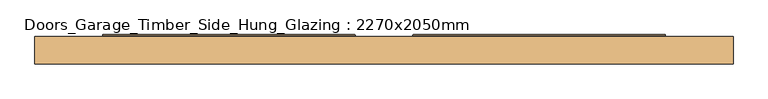
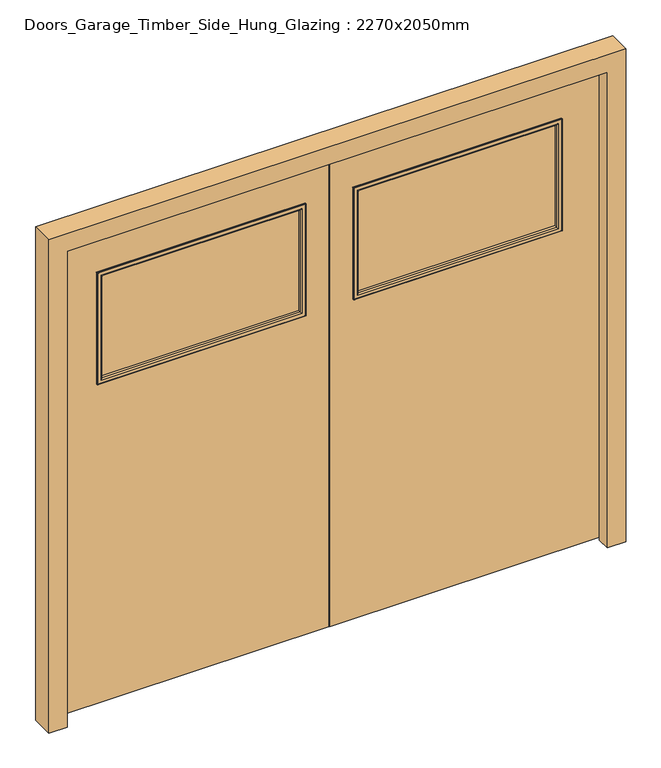
"""IFC4 building model written with IfcOpenShell, lengths in millimetres: door geometry, Doors_Garage_Timber_Side_Hung_Glazing : 2270x2050mm."""

from ifc_helpers import new_model, si_unit, frame, origin, place, context, project, spatial, polyline, ellipse_curve, outline, extrude, faceted_brep, source, transform, mapped, element, save
from ifc_brep_helpers import plane_surface, cylinder_surface, advanced_brep


def doors_garage_timber_side_hung_glazing_2270x2050mm_ae99176d(model_context):
    return source(origin(), model_context, "Body", "SolidModel", [
        faceted_brep([(1085.0, 76.6, 0.0), (1135.0, 76.6, 0.0), (1135.0, -12.4, 0.0), (1063.0, -12.4, 0.0), (1063.0, 41.6, 0.0), (1085.0, 41.6, 0.0), (1085.0, 76.6, 2000.0), (-1085.0, 76.6, 2000.0), (-1085.0, 76.6, 0.0), (-1135.0, 76.6, 0.0), (-1135.0, 76.6, 2050.0), (1135.0, 76.6, 2050.0), (1135.0, -12.4, 2050.0), (-1135.0, -12.4, 2050.0), (-1135.0, -12.4, 0.0), (-1063.0, -12.4, 0.0), (-1063.0, -12.4, 1978.0), (1063.0, -12.4, 1978.0), (1063.0, 41.6, 1978.0), (-1063.0, 41.6, 1978.0), (-1063.0, 41.6, 0.0), (-1085.0, 41.6, 0.0), (-1085.0, 41.6, 2000.0), (1085.0, 41.6, 2000.0)], [[[0, 1, 2, 3, 4, 5]], [[1, 0, 6, 7, 8, 9, 10, 11]], [[2, 1, 11, 12]], [[3, 2, 12, 13, 14, 15, 16, 17]], [[4, 3, 17, 18]], [[5, 4, 18, 19, 20, 21, 22, 23]], [[0, 5, 23, 6]], [[8, 7, 22, 21]], [[9, 8, 21, 20, 15, 14]], [[10, 9, 14, 13]], [[16, 15, 20, 19]], [[11, 10, 13, 12]], [[17, 16, 19, 18]], [[7, 6, 23, 22]]]),
        faceted_brep([(1.5, 44.6, 10.0), (1082.0, 44.6, 10.0), (1082.0, 44.6, 1997.0), (1.5, 44.6, 1997.0), (101.5, 44.6, 1797.0), (907.0, 44.6, 1797.0), (907.0, 44.6, 1347.0), (101.5, 44.6, 1347.0), (1.5, 76.6, 10.0), (1.5, 76.6, 1997.0), (1082.0, 76.6, 1997.0), (1082.0, 76.6, 10.0), (101.5, 76.6, 1797.0), (101.5, 76.6, 1347.0), (907.0, 76.6, 1347.0), (907.0, 76.6, 1797.0), (101.5, 76.6, 1147.0), (101.5, 76.6, 260.0), (907.0, 76.6, 260.0), (907.0, 76.6, 1147.0), (101.5, 71.6, 260.0), (101.5, 71.6, 1147.0), (907.0, 71.6, 1147.0), (907.0, 71.6, 260.0)], [[[0, 1, 2, 3], [4, 5, 6, 7]], [[8, 9, 10, 11], [12, 13, 14, 15], [16, 17, 18, 19]], [[1, 0, 8, 11]], [[2, 1, 11, 10]], [[3, 2, 10, 9]], [[0, 3, 9, 8]], [[5, 4, 12, 15]], [[6, 5, 15, 14]], [[7, 6, 14, 13]], [[4, 7, 13, 12]], [[20, 21, 22, 23]], [[21, 20, 17, 16]], [[22, 21, 16, 19]], [[23, 22, 19, 18]], [[20, 23, 18, 17]]]),
        faceted_brep([(-1082.0, 44.6, 10.0), (-1.5, 44.6, 10.0), (-1.5, 44.6, 1997.0), (-1082.0, 44.6, 1997.0), (-101.5, 44.6, 1347.0), (-907.0, 44.6, 1347.0), (-907.0, 44.6, 1797.0), (-101.5, 44.6, 1797.0), (-1082.0, 76.6, 10.0), (-1082.0, 76.6, 1997.0), (-1.5, 76.6, 1997.0), (-1.5, 76.6, 10.0), (-101.5, 76.6, 1347.0), (-101.5, 76.6, 1797.0), (-907.0, 76.6, 1797.0), (-907.0, 76.6, 1347.0), (-101.5, 76.6, 1147.0), (-907.0, 76.6, 1147.0), (-907.0, 76.6, 260.0), (-101.5, 76.6, 260.0), (-907.0, 71.6, 1147.0), (-101.5, 71.6, 1147.0), (-101.5, 71.6, 260.0), (-907.0, 71.6, 260.0)], [[[0, 1, 2, 3], [4, 5, 6, 7]], [[8, 9, 10, 11], [12, 13, 14, 15], [16, 17, 18, 19]], [[1, 0, 8, 11]], [[2, 1, 11, 10]], [[3, 2, 10, 9]], [[0, 3, 9, 8]], [[5, 4, 12, 15]], [[6, 5, 15, 14]], [[7, 6, 14, 13]], [[4, 7, 13, 12]], [[20, 21, 22, 23]], [[21, 20, 17, 16]], [[22, 21, 16, 19]], [[23, 22, 19, 18]], [[20, 23, 18, 17]]]),
        extrude(outline(polyline([(907.0, 54.6), (101.5, 54.6), (101.5, 66.6), (907.0, 66.6), (907.0, 54.6)])), frame((0.0, 0.0, 1347.0), z_axis=(0.0, 0.0, 1.0), x_axis=(1.0, 0.0, 0.0)), (0.0, 0.0, 1.0), 450.0),
        extrude(outline(polyline([(-101.5, 54.6), (-907.0, 54.6), (-907.0, 66.6), (-101.5, 66.6), (-101.5, 54.6)])), frame((0.0, 0.0, 1347.0), z_axis=(0.0, 0.0, 1.0), x_axis=(1.0, 0.0, 0.0)), (0.0, 0.0, 1.0), 450.0),
        advanced_brep(
        [(-907.0, 66.6, 1797.0), (-907.0, 76.6, 1797.0), (-907.0, 76.6, 1347.0), (-907.0, 66.6, 1347.0), (-895.0, 77.6, 1785.0), (-895.0, 66.6, 1785.0), (-895.0, 66.6, 1359.0), (-895.0, 77.6, 1359.0), (-900.0, 82.6, 1790.0), (-900.0, 82.6, 1354.0), (-915.0, 80.6, 1805.0), (-913.0, 82.6, 1803.0), (-913.0, 82.6, 1341.0), (-915.0, 80.6, 1339.0), (-915.0, 76.6, 1805.0), (-915.0, 76.6, 1339.0), (-101.5, 76.6, 1347.0), (-101.5, 66.6, 1347.0), (-113.5, 66.6, 1359.0), (-113.5, 77.6, 1359.0), (-108.5, 82.6, 1354.0), (-95.5, 82.6, 1341.0), (-93.5, 80.6, 1339.0), (-93.5, 76.6, 1339.0), (-101.5, 76.6, 1797.0), (-101.5, 66.6, 1797.0), (-113.5, 66.6, 1785.0), (-113.5, 77.6, 1785.0), (-108.5, 82.6, 1790.0), (-95.5, 82.6, 1803.0), (-93.5, 80.6, 1805.0), (-93.5, 76.6, 1805.0)],
        [
            (0, 1),
            (1, 2),
            (2, 3),
            (3, 0),
            (4, 5),
            (5, 6),
            (6, 7),
            (7, 4),
            (8, 4, ellipse_curve(frame((-900.0, 77.6, 1790.0), z_axis=(-0.7071067811865475, 0.0, -0.7071067811865475), x_axis=(-0.7071067811865474, 0.0, 0.7071067811865476)), 7.0710678, 5.0)),
            (7, 9, ellipse_curve(frame((-900.0, 77.6, 1354.0), z_axis=(-0.7071067811865475, 0.0, 0.7071067811865475), x_axis=(0.7071067811865474, 0.0, 0.7071067811865476)), 7.0710678, 5.0)),
            (9, 8),
            (10, 11, ellipse_curve(frame((-913.0, 80.6, 1803.0), z_axis=(-0.7071067811865475, 0.0, -0.7071067811865475), x_axis=(-0.7071067811865474, 0.0, 0.7071067811865476)), 2.8284271, 2.0)),
            (11, 12),
            (12, 13, ellipse_curve(frame((-913.0, 80.6, 1341.0), z_axis=(-0.7071067811865475, 0.0, 0.7071067811865475), x_axis=(0.7071067811865474, 0.0, 0.7071067811865476)), 2.8284271, 2.0)),
            (13, 10),
            (14, 10),
            (13, 15),
            (15, 14),
            (2, 16),
            (16, 17),
            (17, 3),
            (6, 18),
            (18, 19),
            (19, 7),
            (19, 20, ellipse_curve(frame((-108.5, 77.6, 1354.0), z_axis=(-0.7071067811865475, 0.0, -0.7071067811865475), x_axis=(-0.7071067811865476, 0.0, 0.7071067811865474)), 7.0710678, 5.0)),
            (20, 9),
            (12, 21),
            (21, 22, ellipse_curve(frame((-95.5, 80.6, 1341.0), z_axis=(-0.7071067811865475, 0.0, -0.7071067811865475), x_axis=(-0.7071067811865476, 0.0, 0.7071067811865474)), 2.8284271, 2.0)),
            (22, 13),
            (22, 23),
            (23, 15),
            (16, 24),
            (24, 25),
            (25, 17),
            (18, 26),
            (26, 27),
            (27, 19),
            (27, 28, ellipse_curve(frame((-108.5, 77.6, 1790.0), z_axis=(0.7071067811865475, 0.0, -0.7071067811865475), x_axis=(-0.7071067811865474, 0.0, -0.7071067811865476)), 7.0710678, 5.0)),
            (28, 20),
            (21, 29),
            (29, 30, ellipse_curve(frame((-95.5, 80.6, 1803.0), z_axis=(0.7071067811865475, 0.0, -0.7071067811865475), x_axis=(-0.7071067811865474, 0.0, -0.7071067811865476)), 2.8284271, 2.0)),
            (30, 22),
            (30, 31),
            (31, 23),
            (31, 14),
            (1, 24),
            (0, 25),
            (5, 26),
            (4, 27),
            (8, 28),
            (11, 29),
            (10, 30),
        ],
        [
            plane_surface(frame((-907.0, 76.6, 1797.0), z_axis=(-1.0, 0.0, 0.0), x_axis=(0.0, 0.0, -1.0))),
            plane_surface(frame((-895.0, 66.6, 1785.0), z_axis=(1.0, 0.0, 0.0), x_axis=(0.0, 0.0, -1.0))),
            cylinder_surface(frame((-900.0, 77.6, 1797.0), z_axis=(0.0, 0.0, 1.0), x_axis=(-1.0, 0.0, 0.0)), 5.0),
            cylinder_surface(frame((-913.0, 80.6, 1797.0), z_axis=(0.0, 0.0, 1.0), x_axis=(-1.0, 0.0, 0.0)), 2.0),
            plane_surface(frame((-915.0, 80.6, 1805.0), z_axis=(-1.0, 0.0, 0.0), x_axis=(0.0, 0.0, -1.0))),
            plane_surface(frame((-907.0, 76.6, 1347.0), z_axis=(0.0, 0.0, -1.0), x_axis=(1.0, 0.0, 0.0))),
            plane_surface(frame((-895.0, 66.6, 1359.0), z_axis=(0.0, 0.0, 1.0), x_axis=(1.0, 0.0, 0.0))),
            cylinder_surface(frame((-907.0, 77.6, 1354.0), z_axis=(-1.0, 0.0, 0.0), x_axis=(0.0, 0.0, -1.0)), 5.0),
            cylinder_surface(frame((-907.0, 80.6, 1341.0), z_axis=(-1.0, 0.0, 0.0), x_axis=(0.0, 0.0, -1.0)), 2.0),
            plane_surface(frame((-915.0, 80.6, 1339.0), z_axis=(0.0, 0.0, -1.0), x_axis=(1.0, 0.0, 0.0))),
            plane_surface(frame((-101.5, 76.6, 1347.0), z_axis=(1.0, 0.0, 0.0), x_axis=(0.0, 0.0, 1.0))),
            plane_surface(frame((-113.5, 66.6, 1359.0), z_axis=(-1.0, 0.0, 0.0), x_axis=(0.0, 0.0, 1.0))),
            cylinder_surface(frame((-108.5, 77.6, 1347.0), z_axis=(0.0, 0.0, -1.0), x_axis=(1.0, 0.0, 0.0)), 5.0),
            cylinder_surface(frame((-95.5, 80.6, 1347.0), z_axis=(0.0, 0.0, -1.0), x_axis=(1.0, 0.0, 0.0)), 2.0),
            plane_surface(frame((-93.5, 80.6, 1339.0), z_axis=(1.0, 0.0, 0.0), x_axis=(0.0, 0.0, 1.0))),
            plane_surface(frame((-93.5, 76.6, 1805.0), z_axis=(0.0, -1.0, 0.0), x_axis=(-1.0, 0.0, 0.0))),
            plane_surface(frame((-101.5, 76.6, 1797.0), z_axis=(0.0, 0.0, 1.0), x_axis=(-1.0, 0.0, 0.0))),
            plane_surface(frame((-101.5, 66.6, 1797.0), z_axis=(0.0, -1.0, 0.0), x_axis=(-1.0, 0.0, 0.0))),
            plane_surface(frame((-113.5, 66.6, 1785.0), z_axis=(0.0, 0.0, -1.0), x_axis=(-1.0, 0.0, 0.0))),
            cylinder_surface(frame((-101.5, 77.6, 1790.0), z_axis=(1.0, 0.0, 0.0), x_axis=(0.0, 0.0, 1.0)), 5.0),
            plane_surface(frame((-108.5, 82.6, 1790.0), z_axis=(0.0, 1.0, 0.0), x_axis=(-1.0, 0.0, 0.0))),
            cylinder_surface(frame((-101.5, 80.6, 1803.0), z_axis=(1.0, 0.0, 0.0), x_axis=(0.0, 0.0, 1.0)), 2.0),
            plane_surface(frame((-93.5, 80.6, 1805.0), z_axis=(0.0, 0.0, 1.0), x_axis=(-1.0, 0.0, 0.0))),
        ],
        [
            (0, [[1, 2, 3, 4]]),
            (1, [[5, 6, 7, 8]]),
            (2, [[9, -8, 10, 11]]),
            (3, [[12, 13, 14, 15]]),
            (4, [[16, -15, 17, 18]]),
            (5, [[-3, 19, 20, 21]]),
            (6, [[-7, 22, 23, 24]]),
            (7, [[-10, -24, 25, 26]]),
            (8, [[-14, 27, 28, 29]]),
            (9, [[-17, -29, 30, 31]]),
            (10, [[-20, 32, 33, 34]]),
            (11, [[-23, 35, 36, 37]]),
            (12, [[-25, -37, 38, 39]]),
            (13, [[-28, 40, 41, 42]]),
            (14, [[-30, -42, 43, 44]]),
            (15, [[-31, -44, 45, -18], [46, -32, -19, -2]]),
            (16, [[-33, -46, -1, 47]]),
            (17, [[-21, -34, -47, -4], [48, -35, -22, -6]]),
            (18, [[-36, -48, -5, 49]]),
            (19, [[-38, -49, -9, 50]]),
            (20, [[51, -40, -27, -13], [-26, -39, -50, -11]]),
            (21, [[-41, -51, -12, 52]]),
            (22, [[-43, -52, -16, -45]]),
        ],
    ),
        advanced_brep(
        [(101.5, 66.6, 1797.0), (101.5, 76.6, 1797.0), (101.5, 76.6, 1347.0), (101.5, 66.6, 1347.0), (113.5, 77.6, 1785.0), (113.5, 66.6, 1785.0), (113.5, 66.6, 1359.0), (113.5, 77.6, 1359.0), (108.5, 82.6, 1790.0), (108.5, 82.6, 1354.0), (93.5, 80.6, 1805.0), (95.5, 82.6, 1803.0), (95.5, 82.6, 1341.0), (93.5, 80.6, 1339.0), (93.5, 76.6, 1805.0), (93.5, 76.6, 1339.0), (907.0, 76.6, 1347.0), (907.0, 66.6, 1347.0), (895.0, 66.6, 1359.0), (895.0, 77.6, 1359.0), (900.0, 82.6, 1354.0), (913.0, 82.6, 1341.0), (915.0, 80.6, 1339.0), (915.0, 76.6, 1339.0), (907.0, 76.6, 1797.0), (907.0, 66.6, 1797.0), (895.0, 66.6, 1785.0), (895.0, 77.6, 1785.0), (900.0, 82.6, 1790.0), (913.0, 82.6, 1803.0), (915.0, 80.6, 1805.0), (915.0, 76.6, 1805.0)],
        [
            (0, 1),
            (1, 2),
            (2, 3),
            (3, 0),
            (4, 5),
            (5, 6),
            (6, 7),
            (7, 4),
            (8, 4, ellipse_curve(frame((108.5, 77.6, 1790.0), z_axis=(-0.7071067811865475, 0.0, -0.7071067811865475), x_axis=(-0.7071067811865474, 0.0, 0.7071067811865476)), 7.0710678, 5.0)),
            (7, 9, ellipse_curve(frame((108.5, 77.6, 1354.0), z_axis=(-0.7071067811865475, 0.0, 0.7071067811865475), x_axis=(0.7071067811865474, 0.0, 0.7071067811865476)), 7.0710678, 5.0)),
            (9, 8),
            (10, 11, ellipse_curve(frame((95.5, 80.6, 1803.0), z_axis=(-0.7071067811865475, 0.0, -0.7071067811865475), x_axis=(-0.7071067811865474, 0.0, 0.7071067811865476)), 2.8284271, 2.0)),
            (11, 12),
            (12, 13, ellipse_curve(frame((95.5, 80.6, 1341.0), z_axis=(-0.7071067811865475, 0.0, 0.7071067811865475), x_axis=(0.7071067811865474, 0.0, 0.7071067811865476)), 2.8284271, 2.0)),
            (13, 10),
            (14, 10),
            (13, 15),
            (15, 14),
            (2, 16),
            (16, 17),
            (17, 3),
            (6, 18),
            (18, 19),
            (19, 7),
            (19, 20, ellipse_curve(frame((900.0, 77.6, 1354.0), z_axis=(-0.7071067811865475, 0.0, -0.7071067811865475), x_axis=(-0.7071067811865476, 0.0, 0.7071067811865474)), 7.0710678, 5.0)),
            (20, 9),
            (12, 21),
            (21, 22, ellipse_curve(frame((913.0, 80.6, 1341.0), z_axis=(-0.7071067811865475, 0.0, -0.7071067811865475), x_axis=(-0.7071067811865476, 0.0, 0.7071067811865474)), 2.8284271, 2.0)),
            (22, 13),
            (22, 23),
            (23, 15),
            (16, 24),
            (24, 25),
            (25, 17),
            (18, 26),
            (26, 27),
            (27, 19),
            (27, 28, ellipse_curve(frame((900.0, 77.6, 1790.0), z_axis=(0.7071067811865475, 0.0, -0.7071067811865475), x_axis=(-0.7071067811865474, 0.0, -0.7071067811865476)), 7.0710678, 5.0)),
            (28, 20),
            (21, 29),
            (29, 30, ellipse_curve(frame((913.0, 80.6, 1803.0), z_axis=(0.7071067811865475, 0.0, -0.7071067811865475), x_axis=(-0.7071067811865474, 0.0, -0.7071067811865476)), 2.8284271, 2.0)),
            (30, 22),
            (30, 31),
            (31, 23),
            (31, 14),
            (1, 24),
            (0, 25),
            (5, 26),
            (4, 27),
            (8, 28),
            (11, 29),
            (10, 30),
        ],
        [
            plane_surface(frame((101.5, 76.6, 1797.0), z_axis=(-1.0, 0.0, 0.0), x_axis=(0.0, 0.0, -1.0))),
            plane_surface(frame((113.5, 66.6, 1785.0), z_axis=(1.0, 0.0, 0.0), x_axis=(0.0, 0.0, -1.0))),
            cylinder_surface(frame((108.5, 77.6, 1797.0), z_axis=(0.0, 0.0, 1.0), x_axis=(-1.0, 0.0, 0.0)), 5.0),
            cylinder_surface(frame((95.5, 80.6, 1797.0), z_axis=(0.0, 0.0, 1.0), x_axis=(-1.0, 0.0, 0.0)), 2.0),
            plane_surface(frame((93.5, 80.6, 1805.0), z_axis=(-1.0, 0.0, 0.0), x_axis=(0.0, 0.0, -1.0))),
            plane_surface(frame((101.5, 76.6, 1347.0), z_axis=(0.0, 0.0, -1.0), x_axis=(1.0, 0.0, 0.0))),
            plane_surface(frame((113.5, 66.6, 1359.0), z_axis=(0.0, 0.0, 1.0), x_axis=(1.0, 0.0, 0.0))),
            cylinder_surface(frame((101.5, 77.6, 1354.0), z_axis=(-1.0, 0.0, 0.0), x_axis=(0.0, 0.0, -1.0)), 5.0),
            cylinder_surface(frame((101.5, 80.6, 1341.0), z_axis=(-1.0, 0.0, 0.0), x_axis=(0.0, 0.0, -1.0)), 2.0),
            plane_surface(frame((93.5, 80.6, 1339.0), z_axis=(0.0, 0.0, -1.0), x_axis=(1.0, 0.0, 0.0))),
            plane_surface(frame((907.0, 76.6, 1347.0), z_axis=(1.0, 0.0, 0.0), x_axis=(0.0, 0.0, 1.0))),
            plane_surface(frame((895.0, 66.6, 1359.0), z_axis=(-1.0, 0.0, 0.0), x_axis=(0.0, 0.0, 1.0))),
            cylinder_surface(frame((900.0, 77.6, 1347.0), z_axis=(0.0, 0.0, -1.0), x_axis=(1.0, 0.0, 0.0)), 5.0),
            cylinder_surface(frame((913.0, 80.6, 1347.0), z_axis=(0.0, 0.0, -1.0), x_axis=(1.0, 0.0, 0.0)), 2.0),
            plane_surface(frame((915.0, 80.6, 1339.0), z_axis=(1.0, 0.0, 0.0), x_axis=(0.0, 0.0, 1.0))),
            plane_surface(frame((915.0, 76.6, 1805.0), z_axis=(0.0, -1.0, 0.0), x_axis=(-1.0, 0.0, 0.0))),
            plane_surface(frame((907.0, 76.6, 1797.0), z_axis=(0.0, 0.0, 1.0), x_axis=(-1.0, 0.0, 0.0))),
            plane_surface(frame((907.0, 66.6, 1797.0), z_axis=(0.0, -1.0, 0.0), x_axis=(-1.0, 0.0, 0.0))),
            plane_surface(frame((895.0, 66.6, 1785.0), z_axis=(0.0, 0.0, -1.0), x_axis=(-1.0, 0.0, 0.0))),
            cylinder_surface(frame((907.0, 77.6, 1790.0), z_axis=(1.0, 0.0, 0.0), x_axis=(0.0, 0.0, 1.0)), 5.0),
            plane_surface(frame((900.0, 82.6, 1790.0), z_axis=(0.0, 1.0, 0.0), x_axis=(-1.0, 0.0, 0.0))),
            cylinder_surface(frame((907.0, 80.6, 1803.0), z_axis=(1.0, 0.0, 0.0), x_axis=(0.0, 0.0, 1.0)), 2.0),
            plane_surface(frame((915.0, 80.6, 1805.0), z_axis=(0.0, 0.0, 1.0), x_axis=(-1.0, 0.0, 0.0))),
        ],
        [
            (0, [[1, 2, 3, 4]]),
            (1, [[5, 6, 7, 8]]),
            (2, [[9, -8, 10, 11]]),
            (3, [[12, 13, 14, 15]]),
            (4, [[16, -15, 17, 18]]),
            (5, [[-3, 19, 20, 21]]),
            (6, [[-7, 22, 23, 24]]),
            (7, [[-10, -24, 25, 26]]),
            (8, [[-14, 27, 28, 29]]),
            (9, [[-17, -29, 30, 31]]),
            (10, [[-20, 32, 33, 34]]),
            (11, [[-23, 35, 36, 37]]),
            (12, [[-25, -37, 38, 39]]),
            (13, [[-28, 40, 41, 42]]),
            (14, [[-30, -42, 43, 44]]),
            (15, [[-31, -44, 45, -18], [46, -32, -19, -2]]),
            (16, [[-33, -46, -1, 47]]),
            (17, [[-21, -34, -47, -4], [48, -35, -22, -6]]),
            (18, [[-36, -48, -5, 49]]),
            (19, [[-38, -49, -9, 50]]),
            (20, [[51, -40, -27, -13], [-26, -39, -50, -11]]),
            (21, [[-41, -51, -12, 52]]),
            (22, [[-43, -52, -16, -45]]),
        ],
    ),
        advanced_brep(
        [(-101.5, 54.6, 1797.0), (-101.5, 44.6, 1797.0), (-101.5, 44.6, 1347.0), (-101.5, 54.6, 1347.0), (-113.5, 43.6, 1785.0), (-113.5, 54.6, 1785.0), (-113.5, 54.6, 1359.0), (-113.5, 43.6, 1359.0), (-108.5, 38.6, 1790.0), (-108.5, 38.6, 1354.0), (-93.5, 40.6, 1805.0), (-95.5, 38.6, 1803.0), (-95.5, 38.6, 1341.0), (-93.5, 40.6, 1339.0), (-93.5, 44.6, 1805.0), (-93.5, 44.6, 1339.0), (-907.0, 44.6, 1347.0), (-907.0, 54.6, 1347.0), (-895.0, 54.6, 1359.0), (-895.0, 43.6, 1359.0), (-900.0, 38.6, 1354.0), (-913.0, 38.6, 1341.0), (-915.0, 40.6, 1339.0), (-915.0, 44.6, 1339.0), (-907.0, 44.6, 1797.0), (-907.0, 54.6, 1797.0), (-895.0, 54.6, 1785.0), (-895.0, 43.6, 1785.0), (-900.0, 38.6, 1790.0), (-913.0, 38.6, 1803.0), (-915.0, 40.6, 1805.0), (-915.0, 44.6, 1805.0)],
        [
            (0, 1),
            (1, 2),
            (2, 3),
            (3, 0),
            (4, 5),
            (5, 6),
            (6, 7),
            (7, 4),
            (8, 4, ellipse_curve(frame((-108.5, 43.6, 1790.0), z_axis=(0.7071067811865525, 0.0, -0.7071067811865426), x_axis=(0.7071067811865425, 0.0, 0.7071067811865525)), 7.0710678, 5.0)),
            (7, 9, ellipse_curve(frame((-108.5, 43.6, 1354.0), z_axis=(0.7071067811865426, 0.0, 0.7071067811865525), x_axis=(-0.7071067811865525, 0.0, 0.7071067811865426)), 7.0710678, 5.0)),
            (9, 8),
            (10, 11, ellipse_curve(frame((-95.5, 40.6, 1803.0), z_axis=(0.7071067811865525, 0.0, -0.7071067811865426), x_axis=(0.7071067811865425, 0.0, 0.7071067811865525)), 2.8284271, 2.0)),
            (11, 12),
            (12, 13, ellipse_curve(frame((-95.5, 40.6, 1341.0), z_axis=(0.7071067811865426, 0.0, 0.7071067811865525), x_axis=(-0.7071067811865525, 0.0, 0.7071067811865426)), 2.8284271, 2.0)),
            (13, 10),
            (14, 10),
            (13, 15),
            (15, 14),
            (2, 16),
            (16, 17),
            (17, 3),
            (6, 18),
            (18, 19),
            (19, 7),
            (19, 20, ellipse_curve(frame((-900.0, 43.6, 1354.0), z_axis=(0.7071067811865527, 0.0, -0.7071067811865422), x_axis=(0.7071067811865424, 0.0, 0.7071067811865527)), 7.0710678, 5.0)),
            (20, 9),
            (12, 21),
            (21, 22, ellipse_curve(frame((-913.0, 40.6, 1341.0), z_axis=(0.7071067811865527, 0.0, -0.7071067811865422), x_axis=(0.7071067811865424, 0.0, 0.7071067811865527)), 2.8284271, 2.0)),
            (22, 13),
            (22, 23),
            (23, 15),
            (16, 24),
            (24, 25),
            (25, 17),
            (18, 26),
            (26, 27),
            (27, 19),
            (27, 28, ellipse_curve(frame((-900.0, 43.6, 1790.0), z_axis=(-0.7071067811865422, 0.0, -0.7071067811865527), x_axis=(0.7071067811865526, 0.0, -0.7071067811865424)), 7.0710678, 5.0)),
            (28, 20),
            (21, 29),
            (29, 30, ellipse_curve(frame((-913.0, 40.6, 1803.0), z_axis=(-0.7071067811865422, 0.0, -0.7071067811865527), x_axis=(0.7071067811865526, 0.0, -0.7071067811865424)), 2.8284271, 2.0)),
            (30, 22),
            (30, 31),
            (31, 23),
            (31, 14),
            (1, 24),
            (0, 25),
            (5, 26),
            (4, 27),
            (8, 28),
            (11, 29),
            (10, 30),
        ],
        [
            plane_surface(frame((-101.5, 44.6, 1797.0), z_axis=(1.0, 0.0, 0.0), x_axis=(0.0, 0.0, -1.0))),
            plane_surface(frame((-113.5, 54.6, 1785.0), z_axis=(-1.0, 0.0, 0.0), x_axis=(0.0, 0.0, -1.0))),
            cylinder_surface(frame((-108.5, 43.6, 1797.0), z_axis=(0.0, 0.0, 1.0), x_axis=(1.0, 0.0, 0.0)), 5.0),
            cylinder_surface(frame((-95.5, 40.6, 1797.0), z_axis=(0.0, 0.0, 1.0), x_axis=(1.0, 0.0, 0.0)), 2.0),
            plane_surface(frame((-93.5, 40.6, 1805.0), z_axis=(1.0, 0.0, 0.0), x_axis=(0.0, 0.0, -1.0))),
            plane_surface(frame((-101.5, 44.6, 1347.0), z_axis=(0.0, 0.0, -1.0), x_axis=(-1.0, 0.0, 0.0))),
            plane_surface(frame((-113.5, 54.6, 1359.0), z_axis=(0.0, 0.0, 1.0), x_axis=(-1.0, 0.0, 0.0))),
            cylinder_surface(frame((-101.5, 43.6, 1354.0), z_axis=(1.0, 0.0, 0.0), x_axis=(0.0, 0.0, -1.0)), 5.0),
            cylinder_surface(frame((-101.5, 40.6, 1341.0), z_axis=(1.0, 0.0, 0.0), x_axis=(0.0, 0.0, -1.0)), 2.0),
            plane_surface(frame((-93.5, 40.6, 1339.0), z_axis=(0.0, 0.0, -1.0), x_axis=(-1.0, 0.0, 0.0))),
            plane_surface(frame((-907.0, 44.6, 1347.0), z_axis=(-1.0, 0.0, 0.0), x_axis=(0.0, 0.0, 1.0))),
            plane_surface(frame((-895.0, 54.6, 1359.0), z_axis=(1.0, 0.0, 0.0), x_axis=(0.0, 0.0, 1.0))),
            cylinder_surface(frame((-900.0, 43.6, 1347.0), z_axis=(0.0, 0.0, -1.0), x_axis=(-1.0, 0.0, 0.0)), 5.0),
            cylinder_surface(frame((-913.0, 40.6, 1347.0), z_axis=(0.0, 0.0, -1.0), x_axis=(-1.0, 0.0, 0.0)), 2.0),
            plane_surface(frame((-915.0, 40.6, 1339.0), z_axis=(-1.0, 0.0, 0.0), x_axis=(0.0, 0.0, 1.0))),
            plane_surface(frame((-915.0, 44.6, 1805.0), z_axis=(0.0, 1.0, 0.0), x_axis=(1.0, 0.0, 0.0))),
            plane_surface(frame((-907.0, 44.6, 1797.0), z_axis=(0.0, 0.0, 1.0), x_axis=(1.0, 0.0, 0.0))),
            plane_surface(frame((-907.0, 54.6, 1797.0), z_axis=(0.0, 1.0, 0.0), x_axis=(1.0, 0.0, 0.0))),
            plane_surface(frame((-895.0, 54.6, 1785.0), z_axis=(0.0, 0.0, -1.0), x_axis=(1.0, 0.0, 0.0))),
            cylinder_surface(frame((-907.0, 43.6, 1790.0), z_axis=(-1.0, 0.0, 0.0), x_axis=(0.0, 0.0, 1.0)), 5.0),
            plane_surface(frame((-900.0, 38.6, 1790.0), z_axis=(0.0, -1.0, 0.0), x_axis=(1.0, 0.0, 0.0))),
            cylinder_surface(frame((-907.0, 40.6, 1803.0), z_axis=(-1.0, 0.0, 0.0), x_axis=(0.0, 0.0, 1.0)), 2.0),
            plane_surface(frame((-915.0, 40.6, 1805.0), z_axis=(0.0, 0.0, 1.0), x_axis=(1.0, 0.0, 0.0))),
        ],
        [
            (0, [[1, 2, 3, 4]]),
            (1, [[5, 6, 7, 8]]),
            (2, [[9, -8, 10, 11]]),
            (3, [[12, 13, 14, 15]]),
            (4, [[16, -15, 17, 18]]),
            (5, [[-3, 19, 20, 21]]),
            (6, [[-7, 22, 23, 24]]),
            (7, [[-10, -24, 25, 26]]),
            (8, [[-14, 27, 28, 29]]),
            (9, [[-17, -29, 30, 31]]),
            (10, [[-20, 32, 33, 34]]),
            (11, [[-23, 35, 36, 37]]),
            (12, [[-25, -37, 38, 39]]),
            (13, [[-28, 40, 41, 42]]),
            (14, [[-30, -42, 43, 44]]),
            (15, [[-31, -44, 45, -18], [46, -32, -19, -2]]),
            (16, [[-33, -46, -1, 47]]),
            (17, [[-21, -34, -47, -4], [48, -35, -22, -6]]),
            (18, [[-36, -48, -5, 49]]),
            (19, [[-38, -49, -9, 50]]),
            (20, [[51, -40, -27, -13], [-26, -39, -50, -11]]),
            (21, [[-41, -51, -12, 52]]),
            (22, [[-43, -52, -16, -45]]),
        ],
    ),
        advanced_brep(
        [(907.0, 54.6, 1797.0), (907.0, 44.6, 1797.0), (907.0, 44.6, 1347.0), (907.0, 54.6, 1347.0), (895.0, 43.6, 1785.0), (895.0, 54.6, 1785.0), (895.0, 54.6, 1359.0), (895.0, 43.6, 1359.0), (900.0, 38.6, 1790.0), (900.0, 38.6, 1354.0), (915.0, 40.6, 1805.0), (913.0, 38.6, 1803.0), (913.0, 38.6, 1341.0), (915.0, 40.6, 1339.0), (915.0, 44.6, 1805.0), (915.0, 44.6, 1339.0), (101.5, 44.6, 1347.0), (101.5, 54.6, 1347.0), (113.5, 54.6, 1359.0), (113.5, 43.6, 1359.0), (108.5, 38.6, 1354.0), (95.5, 38.6, 1341.0), (93.5, 40.6, 1339.0), (93.5, 44.6, 1339.0), (101.5, 44.6, 1797.0), (101.5, 54.6, 1797.0), (113.5, 54.6, 1785.0), (113.5, 43.6, 1785.0), (108.5, 38.6, 1790.0), (95.5, 38.6, 1803.0), (93.5, 40.6, 1805.0), (93.5, 44.6, 1805.0)],
        [
            (0, 1),
            (1, 2),
            (2, 3),
            (3, 0),
            (4, 5),
            (5, 6),
            (6, 7),
            (7, 4),
            (8, 4, ellipse_curve(frame((900.0, 43.6, 1790.0), z_axis=(0.7071067811865528, 0.0, -0.7071067811865421), x_axis=(0.7071067811865421, 0.0, 0.7071067811865529)), 7.0710678, 5.0)),
            (7, 9, ellipse_curve(frame((900.0, 43.6, 1354.0), z_axis=(0.7071067811865421, 0.0, 0.7071067811865528), x_axis=(-0.7071067811865527, 0.0, 0.7071067811865422)), 7.0710678, 5.0)),
            (9, 8),
            (10, 11, ellipse_curve(frame((913.0, 40.6, 1803.0), z_axis=(0.7071067811865528, 0.0, -0.7071067811865421), x_axis=(0.7071067811865421, 0.0, 0.7071067811865529)), 2.8284271, 2.0)),
            (11, 12),
            (12, 13, ellipse_curve(frame((913.0, 40.6, 1341.0), z_axis=(0.7071067811865421, 0.0, 0.7071067811865528), x_axis=(-0.7071067811865527, 0.0, 0.7071067811865422)), 2.8284271, 2.0)),
            (13, 10),
            (14, 10),
            (13, 15),
            (15, 14),
            (2, 16),
            (16, 17),
            (17, 3),
            (6, 18),
            (18, 19),
            (19, 7),
            (19, 20, ellipse_curve(frame((108.5, 43.6, 1354.0), z_axis=(0.7071067811865528, 0.0, -0.7071067811865424), x_axis=(0.7071067811865422, 0.0, 0.7071067811865528)), 7.0710678, 5.0)),
            (20, 9),
            (12, 21),
            (21, 22, ellipse_curve(frame((95.5, 40.6, 1341.0), z_axis=(0.7071067811865528, 0.0, -0.7071067811865424), x_axis=(0.7071067811865422, 0.0, 0.7071067811865528)), 2.8284271, 2.0)),
            (22, 13),
            (22, 23),
            (23, 15),
            (16, 24),
            (24, 25),
            (25, 17),
            (18, 26),
            (26, 27),
            (27, 19),
            (27, 28, ellipse_curve(frame((108.5, 43.6, 1790.0), z_axis=(-0.7071067811865422, 0.0, -0.7071067811865528), x_axis=(0.7071067811865528, 0.0, -0.7071067811865422)), 7.0710678, 5.0)),
            (28, 20),
            (21, 29),
            (29, 30, ellipse_curve(frame((95.5, 40.6, 1803.0), z_axis=(-0.7071067811865422, 0.0, -0.7071067811865528), x_axis=(0.7071067811865528, 0.0, -0.7071067811865422)), 2.8284271, 2.0)),
            (30, 22),
            (30, 31),
            (31, 23),
            (31, 14),
            (1, 24),
            (0, 25),
            (5, 26),
            (4, 27),
            (8, 28),
            (11, 29),
            (10, 30),
        ],
        [
            plane_surface(frame((907.0, 44.6, 1797.0), z_axis=(1.0, 0.0, 0.0), x_axis=(0.0, 0.0, -1.0))),
            plane_surface(frame((895.0, 54.6, 1785.0), z_axis=(-1.0, 0.0, 0.0), x_axis=(0.0, 0.0, -1.0))),
            cylinder_surface(frame((900.0, 43.6, 1797.0), z_axis=(0.0, 0.0, 1.0), x_axis=(1.0, 0.0, 0.0)), 5.0),
            cylinder_surface(frame((913.0, 40.6, 1797.0), z_axis=(0.0, 0.0, 1.0), x_axis=(1.0, 0.0, 0.0)), 2.0),
            plane_surface(frame((915.0, 40.6, 1805.0), z_axis=(1.0, 0.0, 0.0), x_axis=(0.0, 0.0, -1.0))),
            plane_surface(frame((907.0, 44.6, 1347.0), z_axis=(0.0, 0.0, -1.0), x_axis=(-1.0, 0.0, 0.0))),
            plane_surface(frame((895.0, 54.6, 1359.0), z_axis=(0.0, 0.0, 1.0), x_axis=(-1.0, 0.0, 0.0))),
            cylinder_surface(frame((907.0, 43.6, 1354.0), z_axis=(1.0, 0.0, 0.0), x_axis=(0.0, 0.0, -1.0)), 5.0),
            cylinder_surface(frame((907.0, 40.6, 1341.0), z_axis=(1.0, 0.0, 0.0), x_axis=(0.0, 0.0, -1.0)), 2.0),
            plane_surface(frame((915.0, 40.6, 1339.0), z_axis=(0.0, 0.0, -1.0), x_axis=(-1.0, 0.0, 0.0))),
            plane_surface(frame((101.5, 44.6, 1347.0), z_axis=(-1.0, 0.0, 0.0), x_axis=(0.0, 0.0, 1.0))),
            plane_surface(frame((113.5, 54.6, 1359.0), z_axis=(1.0, 0.0, 0.0), x_axis=(0.0, 0.0, 1.0))),
            cylinder_surface(frame((108.5, 43.6, 1347.0), z_axis=(0.0, 0.0, -1.0), x_axis=(-1.0, 0.0, 0.0)), 5.0),
            cylinder_surface(frame((95.5, 40.6, 1347.0), z_axis=(0.0, 0.0, -1.0), x_axis=(-1.0, 0.0, 0.0)), 2.0),
            plane_surface(frame((93.5, 40.6, 1339.0), z_axis=(-1.0, 0.0, 0.0), x_axis=(0.0, 0.0, 1.0))),
            plane_surface(frame((93.5, 44.6, 1805.0), z_axis=(0.0, 1.0, 0.0), x_axis=(1.0, 0.0, 0.0))),
            plane_surface(frame((101.5, 44.6, 1797.0), z_axis=(0.0, 0.0, 1.0), x_axis=(1.0, 0.0, 0.0))),
            plane_surface(frame((101.5, 54.6, 1797.0), z_axis=(0.0, 1.0, 0.0), x_axis=(1.0, 0.0, 0.0))),
            plane_surface(frame((113.5, 54.6, 1785.0), z_axis=(0.0, 0.0, -1.0), x_axis=(1.0, 0.0, 0.0))),
            cylinder_surface(frame((101.5, 43.6, 1790.0), z_axis=(-1.0, 0.0, 0.0), x_axis=(0.0, 0.0, 1.0)), 5.0),
            plane_surface(frame((108.5, 38.6, 1790.0), z_axis=(0.0, -1.0, 0.0), x_axis=(1.0, 0.0, 0.0))),
            cylinder_surface(frame((101.5, 40.6, 1803.0), z_axis=(-1.0, 0.0, 0.0), x_axis=(0.0, 0.0, 1.0)), 2.0),
            plane_surface(frame((93.5, 40.6, 1805.0), z_axis=(0.0, 0.0, 1.0), x_axis=(1.0, 0.0, 0.0))),
        ],
        [
            (0, [[1, 2, 3, 4]]),
            (1, [[5, 6, 7, 8]]),
            (2, [[9, -8, 10, 11]]),
            (3, [[12, 13, 14, 15]]),
            (4, [[16, -15, 17, 18]]),
            (5, [[-3, 19, 20, 21]]),
            (6, [[-7, 22, 23, 24]]),
            (7, [[-10, -24, 25, 26]]),
            (8, [[-14, 27, 28, 29]]),
            (9, [[-17, -29, 30, 31]]),
            (10, [[-20, 32, 33, 34]]),
            (11, [[-23, 35, 36, 37]]),
            (12, [[-25, -37, 38, 39]]),
            (13, [[-28, 40, 41, 42]]),
            (14, [[-30, -42, 43, 44]]),
            (15, [[-31, -44, 45, -18], [46, -32, -19, -2]]),
            (16, [[-33, -46, -1, 47]]),
            (17, [[-21, -34, -47, -4], [48, -35, -22, -6]]),
            (18, [[-36, -48, -5, 49]]),
            (19, [[-38, -49, -9, 50]]),
            (20, [[51, -40, -27, -13], [-26, -39, -50, -11]]),
            (21, [[-41, -51, -12, 52]]),
            (22, [[-43, -52, -16, -45]]),
        ],
    ),
    ])


if __name__ == "__main__":
    model = new_model("IFC4")
    model_context = context("Model", 3, world=origin())
    ifc_project = project(units=[si_unit("LENGTHUNIT", "METRE", prefix="MILLI")], contexts=[model_context])
    site = spatial("IfcSite", under=ifc_project)
    building = spatial("IfcBuilding", under=site)
    placement = place(None, origin())
    doors_garage_timber_side_hung_glazing_2270x2050mm_shape = doors_garage_timber_side_hung_glazing_2270x2050mm_ae99176d(model_context)
    element("IfcDoor", 1, ObjectType="Doors_Garage_Timber_Side_Hung_Glazing : 2270x2050mm", at=placement, inside=building, context=model_context, shape_type="MappedRepresentation", body=[
        mapped(doors_garage_timber_side_hung_glazing_2270x2050mm_shape, transform((0.0, 0.0, 0.0), x_axis=(1.0, 0.0, 0.0), y_axis=(0.0, 1.0, 0.0), z_axis=(0.0, 0.0, 1.0))),
    ])
    save(model, "model.ifc")

# Revit data of these elements
# Type "Doors_Garage_Timber_Side_Hung_Glazing : 2270x2050mm"
#   Type Mark = "8"
#   Type Comments = "External Garage"
#   Operation = "DoubleDoorSingleSwing"
#   Construction Type Id = "GSP4R"
#   Manufacturer = "Revit"
#   Keynote = "L20"
#   Analytic Construction = "1/8 in Pilkington single glazing"
#   Wrap Layers (Ext) from Ext = 0' - 4.03543"
#   Wrap Layers (Int) from Ext = 0' - 6.98819"
#   Visual Light Transmittance = 0.9
#   Thickness = 0' - 1.25984"
#   Stile Top Rail = 0' - 7.87402"
#   Stile Shutting = 0' - 3.93701"
#   Stile Lock Rail = 0' - 7.87402"
#   Stile Hanging = 0' - 6.88976"
#   Stile Bottom Rail = 0' - 9.84252"
#   Solar Heat Gain Coefficient = 0.78
#   Rough Width = 7' - 5.37008"
#   Rough Height = 6' - 8.70866"
#   O/A Frame Width = 0' - 2.51969"
#   Heat Transfer Coefficient (U) = 0.6496 BTU/(h·ft²·°F)
#   Handle Z Distance = 3' - 5.33858"
#   Glazing Panel Height = 1' - 5.71654"
#   FrameWidth = 0' - 1.65354"
#   FrameOffset - External = 0' - 0.98425"
#   FrameDepth = 0' - 3.50394"
#   Door Panel Thickness = 0' - 1.25984"
#   Height = 6' - 8.70866"
#   Structural Tolerance = 0' - 0.31496"
#   Tolerance = 0' - 0.11811"
#   Undercut = 0' - 0.3937"
#   Width = 7' - 5.37008"
#   Cavity Closer Width = 0' - 1.9685"
#   Cavity Closer Offset from Ext = 0' - 4.03543"
#   Cavity Closer Depth = 0' - 3.34646"
#   Vis - Cavity Closers = yes
#   Define Thermal Properties by = 1
#   Function = 1
#   Material Door = Door - Panel
#   Material Frame = Door - Frame/Mullion
#   Material Ironmongery = Door - Handle
#   Wall Closure = (empty or 0)
# Element 1 (IfcDoor, "Doors_Garage_Timber_Side_Hung_Glazing : 2270x2050mm")
#   Materials on its faces: "Door - Panel", "Door - Frame/Mullion", "Door - Glazing"
# Materials
#   "Door - Panel": class "Wood", colour RGB 210 159 95, transparency 0, Cost = 0
#   "Door - Frame/Mullion": class "Wood", colour RGB 212 179 113, transparency 0
#   "Door - Handle": colour RGB 0 0 0, transparency 0
#   "Door - Glazing": colour RGB 0 0 255, transparency 0.75
